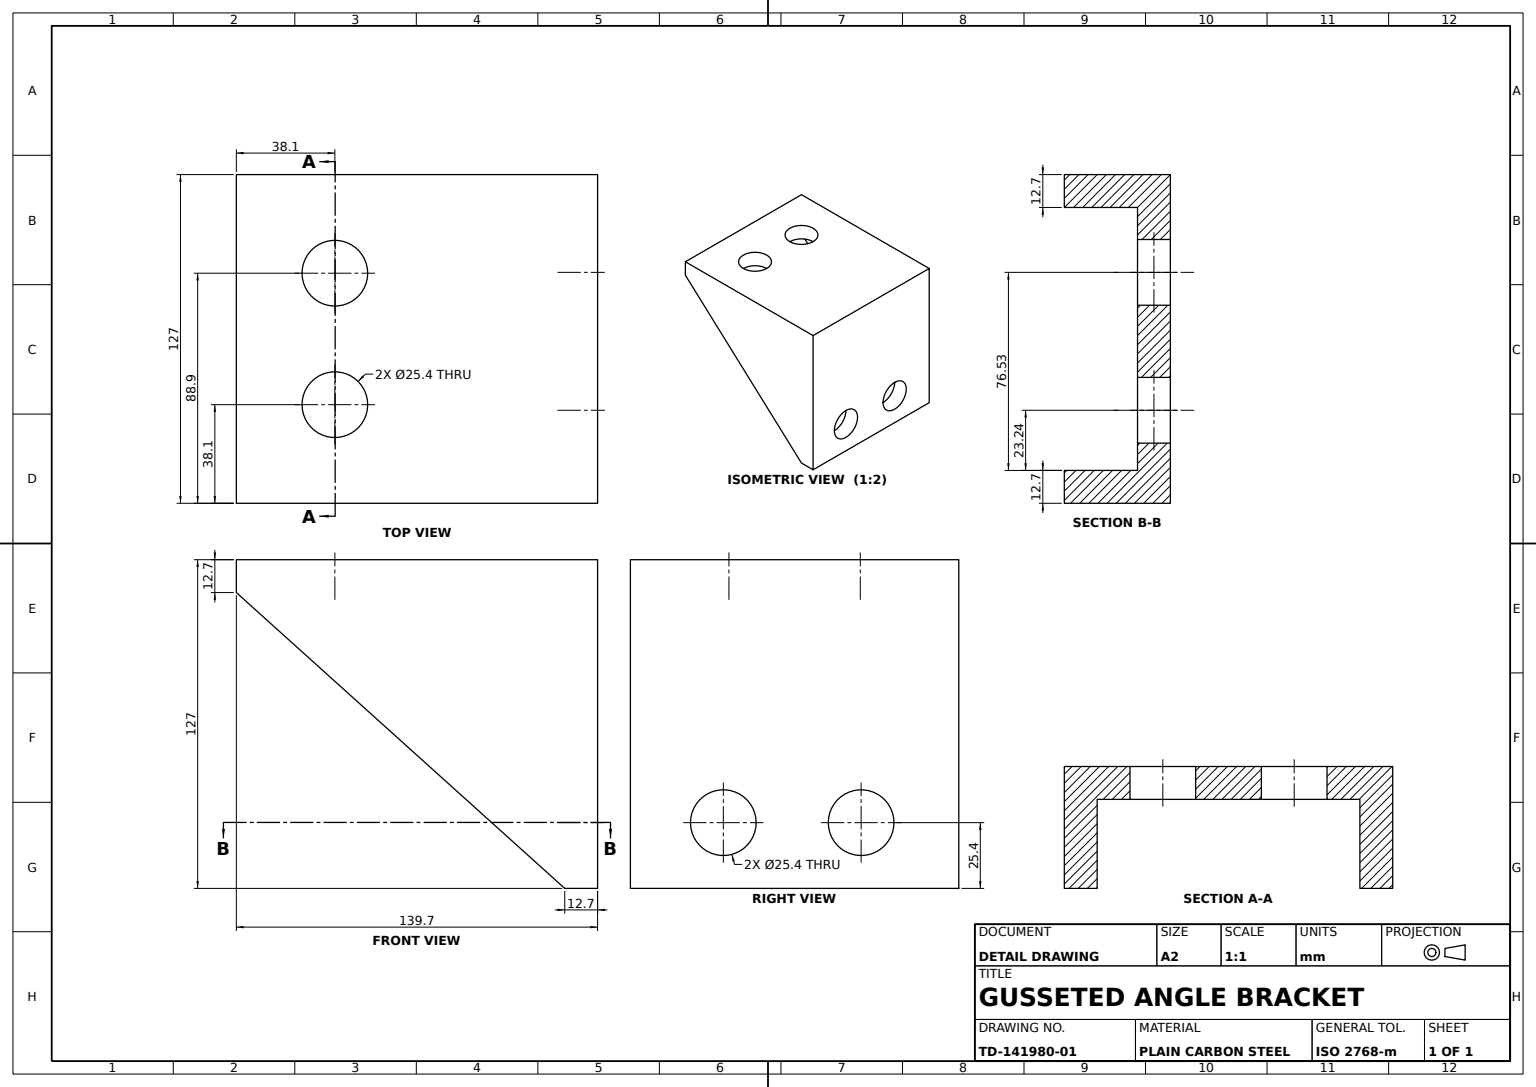
SolidWorks part; units mm, degrees
material "Plain Carbon Steel"
ref_plane "Front Plane" through (0, 0, 0) normal (0, 0, 1) x (1, 0, 0)
ref_plane "Top Plane" through (0, 0, 0) normal (0, 1, 0) x (1, 0, 0)
ref_plane "Right Plane" through (0, 0, 0) normal (1, 0, 0) x (0, 0, -1)
sketch "Base Plate Sketch" plane through (0, 0, 0) normal (0, 0, 1) x (1, 0, 0)
  line L0 (0, 0) -> (0, 127)
  line L1 (0, 127) -> (127, 127)
  line L2 (127, 127) -> (127, 0)
  line L3 (127, 0) -> (0, 0)
  dimension "D1" = 127
  dimension "D2" = 127
  dimension "D3" = 127
  dimension "D4" = 127
extrude "Base Plate" add sketch "Base Plate Sketch" along normal blind 12.7
sketch "Upright Wall Sketch" plane through (0, 0, 12.7) normal (0, 0, 1) x (1, 0, 0)
  line L0 (127, 0) -> (127, 127) construction
  line L1 (0, 127) -> (127, 127)
  line L2 (0, 127) -> (0, 114.3)
  line L3 (0, 114.3) -> (127, 114.3)
  line L4 (127, 127) -> (127, 114.3)
  dimension "D1" = 12.7
extrude "Upright Wall" add sketch "Upright Wall Sketch" along normal blind 127
sketch "Gusset 1 Sketch" plane through (0, 0, 0) normal (-1, 0, 0) x (0, 0, 1)
  line L0 (12.7, 0) -> (139.7, 114.3)
  line L1 (139.7, 114.3) -> (12.7, 114.3)
  line L2 (12.7, 114.3) -> (12.7, 0)
extrude "Gusset 1" add sketch "Gusset 1 Sketch" against normal blind 12.7
sketch "Gusset 2 Sketch" plane through (127, 0, 0) normal (1, 0, 0) x (0, 0, -1)
  line L0 (-12.7, 0) -> (-12.7, 114.3)
  line L1 (-12.7, 114.3) -> (-139.7, 114.3)
  line L2 (-139.7, 114.3) -> (-12.7, 0)
extrude "Gusset 2" add sketch "Gusset 2 Sketch" against normal blind 12.7
sketch "Mounting Hole 1 Sketch" plane through (0, 114.3, 0) normal (0, -1, 0) x (1, 0, 0)
  line L0 (63.5, 139.7) -> (63.5, 12.7)
  line L1 (12.7, 139.7) -> (114.3, 139.7) construction
  line L2 (12.7, 12.7) -> (114.3, 12.7) construction
  circle A0 centre (38.1, 101.6) radius 12.7
  dimension "D1" = 25.4
  dimension "D3" = 25.4
  dimension "D2" = 88.9
extrude "Mounting Hole 1" cut sketch "Mounting Hole 1 Sketch" against normal blind 12.7 contours A0
sketch "Mounting Hole 2 Sketch" plane through (0, 114.3, 0) normal (0, -1, 0) x (1, 0, 0)
  line L0 (12.7, 139.7) -> (114.3, 139.7) construction
  line L1 (12.7, 12.7) -> (114.3, 12.7) construction
  circle A0 centre (88.9, 101.6) radius 12.7
  point P4 (63.5, 139.7)
  dimension "D1" = 25.4
  dimension "D3" = 25.4
  dimension "D2" = 88.9
extrude "Mounting Hole 2" cut sketch "Mounting Hole 2 Sketch" against normal blind 12.7
sketch "Mounting Hole 3 Sketch" plane through (0, 0, 12.7) normal (0, 0, 1) x (1, 0, 0)
  line L0 (12.7, 0) -> (114.3, 0) construction
  line L1 (12.7, 114.3) -> (114.3, 114.3) construction
  line L2 (114.3, 0) -> (114.3, 114.3) construction
  circle A0 centre (37.774, 25.4) radius 12.7
  point P4 (63.5, 0)
  dimension "D1" = 25.4
  dimension "D3" = 25.4
  dimension "D2" = 88.9
  dimension "D4" = 76.526
extrude "Mounting Hole 3" cut sketch "Mounting Hole 3 Sketch" against normal blind 12.7
sketch "Mounting Hole 4 Sketch" plane through (0, 0, 12.7) normal (0, 0, 1) x (1, 0, 0)
  line L0 (12.7, 0) -> (114.3, 0) construction
  line L1 (12.7, 114.3) -> (114.3, 114.3) construction
  line L2 (114.3, 0) -> (114.3, 114.3) construction
  circle A0 centre (91.0636, 25.4) radius 12.7
  dimension "D1" = 25.4
  dimension "D3" = 25.4
  dimension "D2" = 88.9
  dimension "D4" = 23.2364
extrude "Mounting Hole 4" cut sketch "Mounting Hole 4 Sketch" against normal blind 12.7
